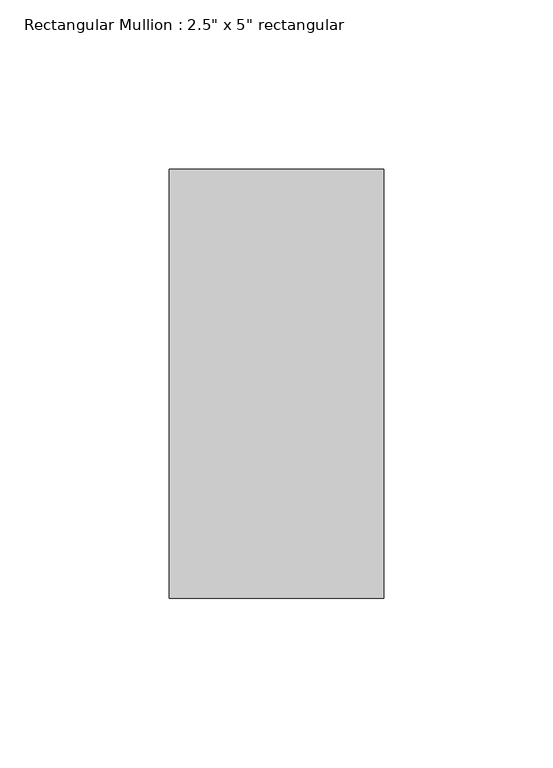
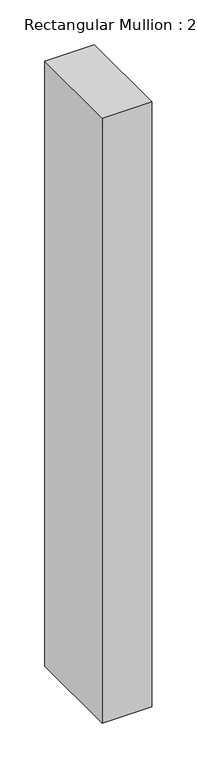
"""IFC4 building model written with IfcOpenShell, lengths in millimetres: member geometry."""

from ifc_helpers import new_model, si_unit, frame, origin, place, context, project, spatial, polyline, outline, extrude, source, transform, mapped, element, save


def member_d7462ea5(model_context):
    return source(origin(), model_context, "Body", "SweptSolid", [
        extrude(outline(polyline([(31.75, 63.5), (31.75, -63.5), (-31.75, -63.5), (-31.75, 63.5), (31.75, 63.5)])), frame((0.0, 0.0, -821.0270145), z_axis=(0.0, 0.0, 1.0), x_axis=(1.0, 0.0, 0.0)), (0.0, 0.0, 1.0), 821.0270145),
    ])


if __name__ == "__main__":
    model = new_model("IFC4")
    model_context = context("Model", 3, world=origin())
    ifc_project = project(units=[si_unit("LENGTHUNIT", "METRE", prefix="MILLI")], contexts=[model_context])
    site = spatial("IfcSite", under=ifc_project)
    building = spatial("IfcBuilding", under=site)
    placement = place(None, origin())
    member_shape = member_d7462ea5(model_context)
    element("IfcMember", 1, ObjectType="Rectangular Mullion : 2.5\" x 5\" rectangular", at=placement, inside=building, context=model_context, shape_type="MappedRepresentation", body=[
        mapped(member_shape, transform((0.0, 0.0, 0.0), x_axis=(1.0, 0.0, 0.0), y_axis=(0.0, 1.0, 0.0), z_axis=(0.0, 0.0, 1.0))),
    ])
    save(model, "model.ifc")

# Revit data of these elements
# Type "Rectangular Mullion : 2.5\" x 5\" rectangular"
#   built-in parameter 1007304 = 0.416667 (stored number, unit not read)
#   built-in parameter 1007301 = 0.104167 (stored number, unit not read)
#   built-in parameter 1007300 = 0.104167 (stored number, unit not read)
# Element 1 (IfcMember, "Rectangular Mullion : 2.5\" x 5\" rectangular")
#   Materials on its faces: "Aluminum"
# Materials
#   "Aluminum": class "Metal", colour RGB 247 247 247, transparency 0, Description = "Aluminum 6061", Cost = 0
